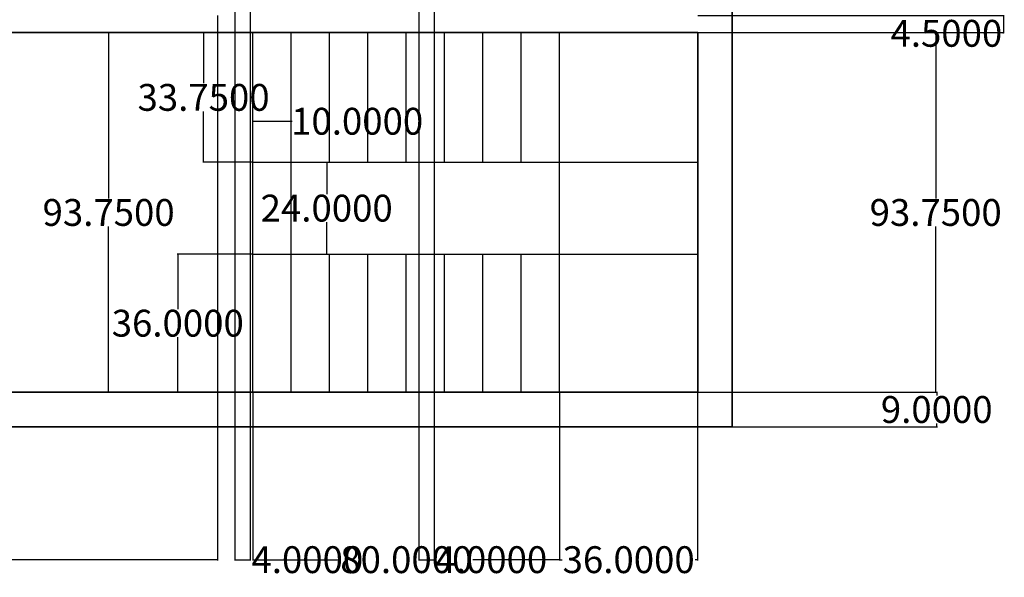
# Model space of a CAD drawing. Units: inches. Extents: x 774 to 2194, y 522 to 1247.
# Tile 2 of 7: x 1035 to 1292, y 522 to 668. Entities that reach past the tile are written whole.
import ezdxf

# ---------------------------------------------------------------- set-up
doc = ezdxf.new("R2010")
doc.units = ezdxf.units.IN
for name, color, linetype, lineweight in [('A-ANNO-DIMS', 2, 'Continuous', 13), ('A-FLOR-STRS', 7, 'Continuous', 25), ('A-WALL', 7, 'Continuous', 35)]:
    doc.layers.add(name, color=color, linetype=linetype, lineweight=lineweight)
doc.styles.get("Standard").update_dxf_attribs({"font": 'arial.ttf'})
doc.dimstyles.get("Standard").update_dxf_attribs({"dimtxt": 7, "dimasz": 0.18, "dimexe": 0.18, "dimexo": 0.0625, "dimgap": 0.09, "dimtad": 0, "dimtih": 1, "dimtoh": 1, "dimdec": 4, "dimzin": 0, "dimdsep": 46, "dimtxsty": 'Standard', "dimcen": 0.09, "dimadec": 0, "dimazin": 0, "dimtfac": 1, "dimtdec": 4, "dimtofl": 0, "dimtmove": 0, "dimatfit": 3, "dimfxl": 1, "dimtolj": 1, "dimtzin": 0, "dimarcsym": 0})

# ---------------------------------------------------------------- blocks, each defined once
blk = doc.blocks.new('*D30')
at = {"layer": 'A-ANNO-DIMS', "color": 0, "lineweight": -2, "transparency": 16777216}
for p, q in [((1211.84, 668.94), (1291.77, 668.94)), ((1291.59, 668.76), (1291.59, 664.62)), ((1211.84, 664.44), (1291.77, 664.44)), ((1291.59, 664.26), (1291.41, 664.26)), ((1291.59, 664.44), (1291.59, 664.26))]:
    blk.add_line(p, q, dxfattribs=at)
at = {"layer": 'A-ANNO-DIMS', "color": 0, "transparency": 16777216}
for points in [[(1291.56, 668.76), (1291.62, 668.76), (1291.59, 668.94)], [(1291.56, 664.62), (1291.62, 664.62), (1291.59, 664.44)]]:
    blk.add_solid(points, dxfattribs=at)
at = {"layer": 'Defpoints', "color": 0, "transparency": 16777216}
for p in [(1211.78, 668.94), (1211.78, 664.44), (1291.59, 664.44)]:
    blk.add_point(p, dxfattribs=at)
at = {"layer": 'A-ANNO-DIMS', "color": 0, "transparency": 16777216, "insert": (1276.66, 664.26), "char_height": 7, "attachment_point": 5}
blk.add_mtext('\\A1;4.5000', dxfattribs=at)
blk = doc.blocks.new('*D31')
at = {"layer": 'A-ANNO-DIMS', "color": 0, "lineweight": -2, "transparency": 16777216}
for p, q in [((1211.84, 664.44), (1274.05, 664.44)), ((1273.87, 664.26), (1273.87, 621.23)), ((1273.87, 570.87), (1273.87, 613.9)), ((1211.84, 570.69), (1274.05, 570.69))]:
    blk.add_line(p, q, dxfattribs=at)
at = {"layer": 'A-ANNO-DIMS', "color": 0, "transparency": 16777216}
for points in [[(1273.84, 664.26), (1273.9, 664.26), (1273.87, 664.44)], [(1273.84, 570.87), (1273.9, 570.87), (1273.87, 570.69)]]:
    blk.add_solid(points, dxfattribs=at)
at = {"layer": 'Defpoints', "color": 0, "transparency": 16777216}
for p in [(1211.78, 664.44), (1211.78, 570.69), (1273.87, 570.69)]:
    blk.add_point(p, dxfattribs=at)
at = {"layer": 'A-ANNO-DIMS', "color": 0, "transparency": 16777216, "insert": (1273.87, 617.56), "char_height": 7, "attachment_point": 5}
blk.add_mtext('\\A1;93.7500', dxfattribs=at)
blk = doc.blocks.new('*D32')
at = {"layer": 'A-ANNO-DIMS', "color": 0, "lineweight": -2, "transparency": 16777216}
for p, q in [((1211.84, 570.69), (1274.32, 570.69)), ((1274.14, 570.51), (1274.14, 569.85)), ((1274.14, 561.87), (1274.14, 562.52)), ((1211.84, 561.69), (1274.32, 561.69))]:
    blk.add_line(p, q, dxfattribs=at)
at = {"layer": 'A-ANNO-DIMS', "color": 0, "transparency": 16777216}
for points in [[(1274.11, 570.51), (1274.17, 570.51), (1274.14, 570.69)], [(1274.11, 561.87), (1274.17, 561.87), (1274.14, 561.69)]]:
    blk.add_solid(points, dxfattribs=at)
at = {"layer": 'Defpoints', "color": 0, "transparency": 16777216}
for p in [(1211.78, 570.69), (1211.78, 561.69), (1274.14, 561.69)]:
    blk.add_point(p, dxfattribs=at)
at = {"layer": 'A-ANNO-DIMS', "color": 0, "transparency": 16777216, "insert": (1274.14, 566.19), "char_height": 7, "attachment_point": 5}
blk.add_mtext('\\A1;9.0000', dxfattribs=at)
blk = doc.blocks.new('*D33')
at = {"layer": 'A-ANNO-DIMS', "color": 0, "lineweight": -2, "transparency": 16777216}
for p, q in [((1095.72, 664.44), (1057.94, 664.44)), ((1058.12, 664.26), (1058.12, 621.23)), ((1058.12, 570.87), (1058.12, 613.9)), ((1095.72, 570.69), (1057.94, 570.69))]:
    blk.add_line(p, q, dxfattribs=at)
at = {"layer": 'A-ANNO-DIMS', "color": 0, "transparency": 16777216}
for points in [[(1058.09, 664.26), (1058.15, 664.26), (1058.12, 664.44)], [(1058.09, 570.87), (1058.15, 570.87), (1058.12, 570.69)]]:
    blk.add_solid(points, dxfattribs=at)
at = {"layer": 'Defpoints', "color": 0, "transparency": 16777216}
for p in [(1095.78, 664.44), (1058.12, 570.69), (1095.78, 570.69)]:
    blk.add_point(p, dxfattribs=at)
at = {"layer": 'A-ANNO-DIMS', "color": 0, "transparency": 16777216, "insert": (1058.12, 617.56), "char_height": 7, "attachment_point": 5}
blk.add_mtext('\\A1;93.7500', dxfattribs=at)
blk = doc.blocks.new('*D34')
at = {"layer": 'A-ANNO-DIMS', "color": 0, "lineweight": -2, "transparency": 16777216}
for p, q in [((1095.72, 664.44), (1082.71, 664.44)), ((1082.89, 664.26), (1082.89, 651.23)), ((1082.89, 630.87), (1082.89, 643.9)), ((1095.72, 630.69), (1082.71, 630.69))]:
    blk.add_line(p, q, dxfattribs=at)
at = {"layer": 'A-ANNO-DIMS', "color": 0, "transparency": 16777216}
for points in [[(1082.86, 664.26), (1082.92, 664.26), (1082.89, 664.44)], [(1082.86, 630.87), (1082.92, 630.87), (1082.89, 630.69)]]:
    blk.add_solid(points, dxfattribs=at)
at = {"layer": 'Defpoints', "color": 0, "transparency": 16777216}
for p in [(1082.89, 664.44), (1095.78, 664.44), (1095.78, 630.69)]:
    blk.add_point(p, dxfattribs=at)
at = {"layer": 'A-ANNO-DIMS', "color": 0, "transparency": 16777216, "insert": (1082.89, 647.56), "char_height": 7, "attachment_point": 5}
blk.add_mtext('\\A1;33.7500', dxfattribs=at)
blk = doc.blocks.new('*D35')
at = {"layer": 'A-ANNO-DIMS', "color": 0, "lineweight": -2, "transparency": 16777216}
for p, q in [((1095.72, 606.69), (1075.98, 606.69)), ((1076.16, 606.51), (1076.16, 592.35)), ((1076.16, 570.87), (1076.16, 585.02)), ((1095.72, 570.69), (1075.98, 570.69))]:
    blk.add_line(p, q, dxfattribs=at)
at = {"layer": 'A-ANNO-DIMS', "color": 0, "transparency": 16777216}
for points in [[(1076.13, 606.51), (1076.19, 606.51), (1076.16, 606.69)], [(1076.13, 570.87), (1076.19, 570.87), (1076.16, 570.69)]]:
    blk.add_solid(points, dxfattribs=at)
at = {"layer": 'Defpoints', "color": 0, "transparency": 16777216}
for p in [(1095.78, 606.69), (1076.16, 570.69), (1095.78, 570.69)]:
    blk.add_point(p, dxfattribs=at)
at = {"layer": 'A-ANNO-DIMS', "color": 0, "transparency": 16777216, "insert": (1076.16, 588.69), "char_height": 7, "attachment_point": 5}
blk.add_mtext('\\A1;36.0000', dxfattribs=at)
blk = doc.blocks.new('*D36')
at = {"layer": 'A-ANNO-DIMS', "color": 0, "lineweight": -2, "transparency": 16777216}
for p, q in [((1095.84, 630.69), (1115.19, 630.69)), ((1115.01, 630.51), (1115.01, 622.35)), ((1115.01, 606.87), (1115.01, 615.02)), ((1095.84, 606.69), (1115.19, 606.69))]:
    blk.add_line(p, q, dxfattribs=at)
at = {"layer": 'A-ANNO-DIMS', "color": 0, "transparency": 16777216}
for points in [[(1114.98, 630.51), (1115.04, 630.51), (1115.01, 630.69)], [(1114.98, 606.87), (1115.04, 606.87), (1115.01, 606.69)]]:
    blk.add_solid(points, dxfattribs=at)
at = {"layer": 'Defpoints', "color": 0, "transparency": 16777216}
for p in [(1095.78, 630.69), (1095.78, 606.69), (1115.01, 606.69)]:
    blk.add_point(p, dxfattribs=at)
at = {"layer": 'A-ANNO-DIMS', "color": 0, "transparency": 16777216, "insert": (1115.01, 618.69), "char_height": 7, "attachment_point": 5}
blk.add_mtext('\\A1;24.0000', dxfattribs=at)
blk = doc.blocks.new('*D51')
at = {"layer": 'A-ANNO-DIMS', "color": 0, "lineweight": -2, "transparency": 16777216}
for p, q in [((1095.78, 570.63), (1095.78, 526.86)), ((1175.78, 570.63), (1175.78, 526.86)), ((1095.96, 527.04), (1118.45, 527.04)), ((1175.6, 527.04), (1153.11, 527.04))]:
    blk.add_line(p, q, dxfattribs=at)
at = {"layer": 'A-ANNO-DIMS', "color": 0, "transparency": 16777216}
for points in [[(1095.96, 527.07), (1095.96, 527.01), (1095.78, 527.04)], [(1175.6, 527.07), (1175.6, 527.01), (1175.78, 527.04)]]:
    blk.add_solid(points, dxfattribs=at)
at = {"layer": 'Defpoints', "color": 0, "transparency": 16777216}
for p in [(1095.78, 570.69), (1175.78, 570.69), (1175.78, 527.04)]:
    blk.add_point(p, dxfattribs=at)
at = {"layer": 'A-ANNO-DIMS', "color": 0, "transparency": 16777216, "insert": (1135.78, 527.04), "char_height": 7, "attachment_point": 5}
blk.add_mtext('\\A1;80.0000', dxfattribs=at)
blk = doc.blocks.new('*D52')
at = {"layer": 'A-ANNO-DIMS', "color": 0, "lineweight": -2, "transparency": 16777216}
for p, q in [((1095.78, 606.75), (1095.78, 641.52)), ((1095.96, 641.34), (1105.6, 641.34)), ((1105.78, 606.75), (1105.78, 641.52)), ((1105.78, 641.34), (1105.96, 641.34))]:
    blk.add_line(p, q, dxfattribs=at)
at = {"layer": 'A-ANNO-DIMS', "color": 0, "transparency": 16777216}
for points in [[(1095.96, 641.37), (1095.96, 641.31), (1095.78, 641.34)], [(1105.6, 641.37), (1105.6, 641.31), (1105.78, 641.34)]]:
    blk.add_solid(points, dxfattribs=at)
at = {"layer": 'Defpoints', "color": 0, "transparency": 16777216}
for p in [(1105.78, 641.34), (1095.78, 606.69), (1105.78, 606.69)]:
    blk.add_point(p, dxfattribs=at)
at = {"layer": 'A-ANNO-DIMS', "color": 0, "transparency": 16777216, "insert": (1122.96, 641.34), "char_height": 7, "attachment_point": 5}
blk.add_mtext('\\A1;10.0000', dxfattribs=at)
blk = doc.blocks.new('*D53')
at = {"layer": 'A-ANNO-DIMS', "color": 0, "lineweight": -2, "transparency": 16777216}
for p, q in [((1175.78, 570.63), (1175.78, 526.86)), ((1211.78, 570.63), (1211.78, 526.86)), ((1175.96, 527.04), (1176.46, 527.04)), ((1211.6, 527.04), (1211.11, 527.04))]:
    blk.add_line(p, q, dxfattribs=at)
at = {"layer": 'A-ANNO-DIMS', "color": 0, "transparency": 16777216}
for points in [[(1175.96, 527.07), (1175.96, 527.01), (1175.78, 527.04)], [(1211.6, 527.07), (1211.6, 527.01), (1211.78, 527.04)]]:
    blk.add_solid(points, dxfattribs=at)
at = {"layer": 'Defpoints', "color": 0, "transparency": 16777216}
for p in [(1175.78, 570.69), (1211.78, 570.69), (1211.78, 527.04)]:
    blk.add_point(p, dxfattribs=at)
at = {"layer": 'A-ANNO-DIMS', "color": 0, "transparency": 16777216, "insert": (1193.78, 527.04), "char_height": 7, "attachment_point": 5}
blk.add_mtext('\\A1;36.0000', dxfattribs=at)
blk = doc.blocks.new('*D55')
at = {"layer": 'A-ANNO-DIMS', "color": 0, "lineweight": -2, "transparency": 16777216}
for p, q in [((869.78, 668.88), (869.78, 526.86)), ((1086.53, 668.88), (1086.53, 526.86)), ((869.96, 527.04), (958.05, 527.04)), ((1086.35, 527.04), (998.26, 527.04))]:
    blk.add_line(p, q, dxfattribs=at)
at = {"layer": 'A-ANNO-DIMS', "color": 0, "transparency": 16777216}
for points in [[(869.96, 527.07), (869.96, 527.01), (869.78, 527.04)], [(1086.35, 527.07), (1086.35, 527.01), (1086.53, 527.04)]]:
    blk.add_solid(points, dxfattribs=at)
at = {"layer": 'Defpoints', "color": 0, "transparency": 16777216}
for p in [(869.78, 668.94), (1086.53, 668.94), (1086.53, 527.04)]:
    blk.add_point(p, dxfattribs=at)
at = {"layer": 'A-ANNO-DIMS', "color": 0, "transparency": 16777216, "insert": (978.16, 527.04), "char_height": 7, "attachment_point": 5}
blk.add_mtext('\\A1;216.7500', dxfattribs=at)
blk = doc.blocks.new('*D71')
at = {"layer": 'A-ANNO-DIMS', "color": 0, "lineweight": -2, "transparency": 16777216}
for p, q in [((1139.03, 812.87), (1139.03, 526.86)), ((1143.03, 812.87), (1143.03, 526.86)), ((1139.21, 527.04), (1142.85, 527.04)), ((1143.03, 527.04), (1143.21, 527.04))]:
    blk.add_line(p, q, dxfattribs=at)
at = {"layer": 'A-ANNO-DIMS', "color": 0, "transparency": 16777216}
for points in [[(1139.21, 527.07), (1139.21, 527.01), (1139.03, 527.04)], [(1142.85, 527.07), (1142.85, 527.01), (1143.03, 527.04)]]:
    blk.add_solid(points, dxfattribs=at)
at = {"layer": 'Defpoints', "color": 0, "transparency": 16777216}
for p in [(1139.03, 812.94), (1143.03, 812.94), (1143.03, 527.04)]:
    blk.add_point(p, dxfattribs=at)
at = {"layer": 'A-ANNO-DIMS', "color": 0, "transparency": 16777216, "insert": (1157.96, 527.04), "char_height": 7, "attachment_point": 5}
blk.add_mtext('\\A1;4.0000', dxfattribs=at)
blk = doc.blocks.new('*D74')
at = {"layer": 'A-ANNO-DIMS', "color": 0, "lineweight": -2, "transparency": 16777216}
for p, q in [((1091.03, 808.38), (1091.03, 526.86)), ((1095.03, 808.38), (1095.03, 526.86)), ((1091.21, 527.04), (1094.85, 527.04)), ((1095.03, 527.04), (1095.21, 527.04))]:
    blk.add_line(p, q, dxfattribs=at)
at = {"layer": 'A-ANNO-DIMS', "color": 0, "transparency": 16777216}
for points in [[(1091.21, 527.07), (1091.21, 527.01), (1091.03, 527.04)], [(1094.85, 527.07), (1094.85, 527.01), (1095.03, 527.04)]]:
    blk.add_solid(points, dxfattribs=at)
at = {"layer": 'Defpoints', "color": 0, "transparency": 16777216}
for p in [(1091.03, 808.44), (1095.03, 808.44), (1095.03, 527.04)]:
    blk.add_point(p, dxfattribs=at)
at = {"layer": 'A-ANNO-DIMS', "color": 0, "transparency": 16777216, "insert": (1109.96, 527.04), "char_height": 7, "attachment_point": 5}
blk.add_mtext('\\A1;4.0000', dxfattribs=at)

msp = doc.modelspace()

# ---------------------------------------------------------------- linework, layer by layer
at = {"layer": 'A-FLOR-STRS'}
for p, q in [((1095.78103, 570.6875), (1095.78103, 664.4375)), ((1105.78103, 630.6875), (1105.78103, 664.4375)), ((1105.78103, 630.6875), (1105.78103, 664.4375)), ((1115.78103, 630.6875), (1115.78103, 664.4375)), ((1115.78103, 630.6875), (1115.78103, 664.4375)), ((1125.78103, 630.6875), (1125.78103, 664.4375)), ((1125.78103, 630.6875), (1125.78103, 664.4375)), ((1135.78103, 630.6875), (1135.78103, 664.4375)), ((1135.78103, 630.6875), (1135.78103, 664.4375)), ((1145.78103, 630.6875), (1145.78103, 664.4375)), ((1145.78103, 630.6875), (1145.78103, 664.4375)), ((1155.78103, 630.6875), (1155.78103, 664.4375)), ((1155.78103, 630.6875), (1155.78103, 664.4375)), ((1165.78103, 630.6875), (1165.78103, 664.4375)), ((1165.78103, 630.6875), (1165.78103, 664.4375)), ((1175.78103, 570.6875), (1175.78103, 664.4375)), ((1211.78103, 570.6875), (1211.78103, 664.4375)), ((1095.78103, 630.6875), (1211.78103, 630.6875)), ((1095.78103, 606.6875), (1211.78103, 606.6875)), ((1105.78103, 570.6875), (1105.78103, 606.6875)), ((1105.78103, 570.6875), (1105.78103, 606.6875)), ((1115.78103, 570.6875), (1115.78103, 606.6875)), ((1115.78103, 570.6875), (1115.78103, 606.6875)), ((1125.78103, 570.6875), (1125.78103, 606.6875)), ((1125.78103, 570.6875), (1125.78103, 606.6875)), ((1135.78103, 570.6875), (1135.78103, 606.6875)), ((1135.78103, 570.6875), (1135.78103, 606.6875)), ((1145.78103, 570.6875), (1145.78103, 606.6875)), ((1145.78103, 570.6875), (1145.78103, 606.6875)), ((1155.78103, 570.6875), (1155.78103, 606.6875)), ((1155.78103, 570.6875), (1155.78103, 606.6875)), ((1165.78103, 570.6875), (1165.78103, 606.6875)), ((1165.78103, 570.6875), (1165.78103, 606.6875)), ((1088.78103, 570.6875), (1211.78103, 570.6875))]:
    msp.add_line(p, q, dxfattribs=at)
at = {"layer": 'A-WALL'}
for p, q in [((1220.78103, 570.6875), (1220.78103, 1050.6875)), ((1220.78103, 666.6875), (1220.78103, 561.6875)), ((1010.53103, 664.4375), (1211.78103, 664.4375)), ((1211.78103, 570.6875), (1211.78103, 664.4375)), ((1014.53103, 570.6875), (1211.78103, 570.6875)), ((1014.53103, 561.6875), (1220.78103, 561.6875))]:
    msp.add_line(p, q, dxfattribs=at)

# ---------------------------------------------------------------- dimensions: what is measured, and where the dimension line sits
at = {"layer": 'A-ANNO-DIMS'}
for base, p1, p2, picture, middle in [((1143.03103, 527.0375), (1139.03103, 812.93598), (1143.03103, 812.93598), '*D71', (1157.95996, 527.0375)), ((1095.03103, 527.0375), (1091.03103, 808.4375), (1095.03103, 808.4375), '*D74', (1109.95996, 527.0375)), ((1086.53103, 527.0375), (869.78103, 668.9375), (1086.53103, 668.9375), '*D55', (978.15603, 527.0375)), ((1105.78103, 641.3375), (1095.78103, 606.6875), (1105.78103, 606.6875), '*D52', (1122.95894, 641.3375)), ((1175.78103, 527.0375), (1095.78103, 570.6875), (1175.78103, 570.6875), '*D51', (1135.78103, 527.0375)), ((1211.78103, 527.0375), (1175.78103, 570.6875), (1211.78103, 570.6875), '*D53', (1193.78103, 527.0375))]:
    dim = msp.add_linear_dim(base=base, p1=p1, p2=p2, dimstyle='Standard', override={"dimdec": 4, "dimlfac": 1, "dimrnd": 0, "dimzin": 0, "dimdsep": 46, "dimlunit": 2}, dxfattribs=at)
    dim.commit()
    dim.dimension.update_dxf_attribs({"geometry": picture, "text_midpoint": middle})
for base, p1, p2, picture, middle in [((1291.5904, 664.4375), (1211.78103, 668.9375), (1211.78103, 664.4375), '*D30', (1276.66146, 664.2575)), ((1058.11548, 570.6875), (1095.78103, 664.4375), (1095.78103, 570.6875), '*D33', (1058.11548, 617.5625)), ((1082.89205, 664.4375), (1095.78103, 630.6875), (1095.78103, 664.4375), '*D34', (1082.89205, 647.5625)), ((1273.87241, 570.6875), (1211.78103, 664.4375), (1211.78103, 570.6875), '*D31', (1273.87241, 617.5625)), ((1115.00981, 606.6875), (1095.78103, 630.6875), (1095.78103, 606.6875), '*D36', (1115.00981, 618.6875)), ((1076.1626, 570.6875), (1095.78103, 606.6875), (1095.78103, 570.6875), '*D35', (1076.1626, 588.6875)), ((1274.14492, 561.6875), (1211.78103, 570.6875), (1211.78103, 561.6875), '*D32', (1274.14492, 566.1875))]:
    dim = msp.add_linear_dim(base=base, p1=p1, p2=p2, angle=90, dimstyle='Standard', override={"dimclrd": 0, "dimclre": 0, "dimclrt": 0}, dxfattribs=at)
    dim.commit()
    dim.dimension.update_dxf_attribs({"geometry": picture, "text_midpoint": middle})

doc.saveas('drawing.dxf')
